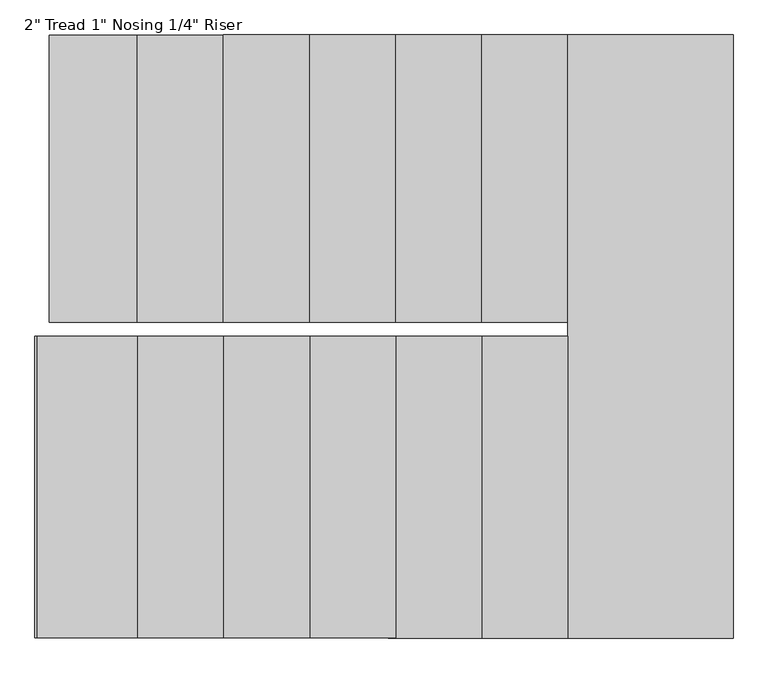
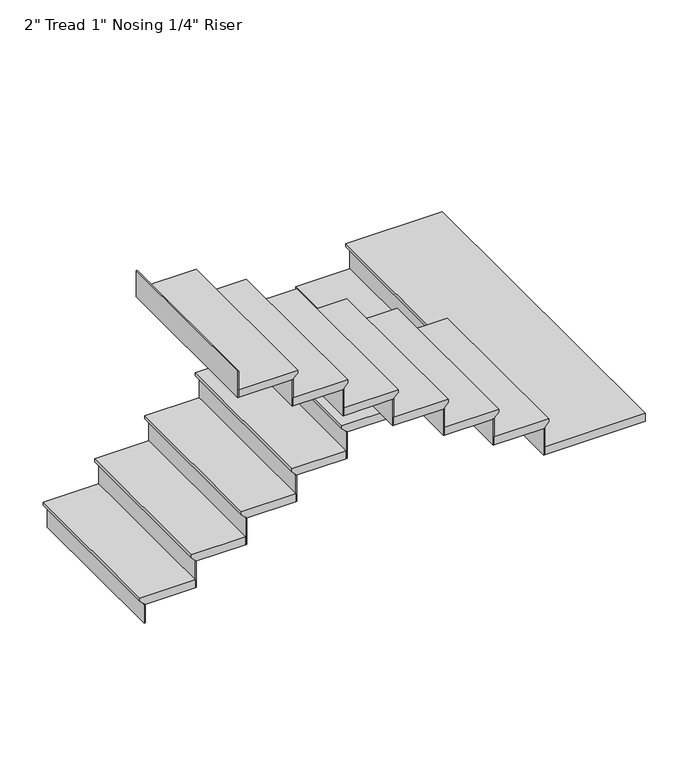
"""IFC4 building model written with IfcOpenShell, lengths in millimetres: stair flight geometry."""

from ifc_helpers import new_model, si_unit, origin, place, context, project, spatial, faceted_brep, source, transform, mapped, element, save


def stair_flight_cd9d6a89(model_context):
    return source(origin(), model_context, "Body", "Brep", [
        faceted_brep([(-1167.6638307, -167.7482799, 9751.4833333), (-1167.6638307, -167.7482799, 9770.5333333), (-1167.6638307, 848.2517201, 9770.5333333), (-1167.6638307, 848.2517201, 9751.4833333), (-1142.2638307, -167.7482799, 9726.0833333), (-1142.2638307, 848.2517201, 9726.0833333), (-831.1138307, -167.7482799, 9770.5333333), (-831.1138307, 848.2517201, 9770.5333333), (-1142.2638307, 848.2517201, 9719.7333333), (-831.1138307, 848.2517201, 9719.7333333), (-831.1138307, -167.7482799, 9719.7333333), (-1142.2638307, -167.7482799, 9719.7333333)], [[[0, 1, 2, 3]], [[4, 0, 3, 5]], [[2, 1, 6, 7]], [[8, 9, 10, 11]], [[2, 7, 9, 8, 5, 3]], [[8, 11, 4, 5]], [[6, 1, 0, 4, 11, 10]], [[7, 6, 10, 9]]]),
        faceted_brep([(-1142.2638307, -167.7482799, 9719.7333333), (-1142.2638307, -167.7482799, 9601.2), (-1135.9138307, -167.7482799, 9601.2), (-1135.9138307, -167.7482799, 9719.7333333), (-1142.2638307, 848.2517201, 9719.7333333), (-1135.9138307, 848.2517201, 9719.7333333), (-1135.9138307, 848.2517201, 9601.2), (-1142.2638307, 848.2517201, 9601.2)], [[[0, 1, 2, 3]], [[4, 5, 6, 7]], [[1, 0, 4, 7]], [[2, 1, 7, 6]], [[3, 2, 6, 5]], [[0, 3, 5, 4]]]),
        faceted_brep([(-831.1138307, -167.7482799, 9889.0666667), (-831.1138307, -167.7482799, 9719.7333333), (-824.7638307, -167.7482799, 9719.7333333), (-824.7638307, -167.7482799, 9889.0666667), (-831.1138307, 848.2517201, 9889.0666667), (-824.7638307, 848.2517201, 9889.0666667), (-824.7638307, 848.2517201, 9719.7333333), (-831.1138307, 848.2517201, 9719.7333333)], [[[0, 1, 2, 3]], [[4, 5, 6, 7]], [[1, 0, 4, 7]], [[2, 1, 7, 6]], [[3, 2, 6, 5]], [[0, 3, 5, 4]]]),
        faceted_brep([(-856.5138307, 848.2517201, 9939.8666667), (-856.5138307, -167.7482799, 9939.8666667), (-526.3138307, -167.7482799, 9939.8666667), (-526.3138307, 848.2517201, 9939.8666667), (-831.1138307, 848.2517201, 9889.0666667), (-526.3138307, 848.2517201, 9889.0666667), (-526.3138307, -167.7482799, 9889.0666667), (-831.1138307, -167.7482799, 9889.0666667), (-831.1138307, 848.2517201, 9895.4166667), (-856.5138307, 848.2517201, 9920.8166667), (-831.1138307, -167.7482799, 9895.4166667), (-856.5138307, -167.7482799, 9920.8166667)], [[[0, 1, 2, 3]], [[4, 5, 6, 7]], [[0, 3, 5, 4, 8, 9]], [[4, 7, 10, 8]], [[2, 1, 11, 10, 7, 6]], [[3, 2, 6, 5]], [[11, 1, 0, 9]], [[10, 11, 9, 8]]]),
        faceted_brep([(-526.3138307, -167.7482799, 10058.4), (-526.3138307, -167.7482799, 9889.0666667), (-519.9638307, -167.7482799, 9889.0666667), (-519.9638307, -167.7482799, 10058.4), (-526.3138307, 848.2517201, 10058.4), (-519.9638307, 848.2517201, 10058.4), (-519.9638307, 848.2517201, 9889.0666667), (-526.3138307, 848.2517201, 9889.0666667)], [[[0, 1, 2, 3]], [[4, 5, 6, 7]], [[1, 0, 4, 7]], [[2, 1, 7, 6]], [[3, 2, 6, 5]], [[0, 3, 5, 4]]]),
        faceted_brep([(-551.7138307, 848.2517201, 10109.2), (-551.7138307, -167.7482799, 10109.2), (-221.5138307, -167.7482799, 10109.2), (-221.5138307, 848.2517201, 10109.2), (-526.3138307, 848.2517201, 10058.4), (-221.5138307, 848.2517201, 10058.4), (-221.5138307, -167.7482799, 10058.4), (-526.3138307, -167.7482799, 10058.4), (-526.3138307, 848.2517201, 10064.75), (-551.7138307, 848.2517201, 10090.15), (-526.3138307, -167.7482799, 10064.75), (-551.7138307, -167.7482799, 10090.15)], [[[0, 1, 2, 3]], [[4, 5, 6, 7]], [[0, 3, 5, 4, 8, 9]], [[4, 7, 10, 8]], [[2, 1, 11, 10, 7, 6]], [[3, 2, 6, 5]], [[11, 1, 0, 9]], [[10, 11, 9, 8]]]),
        faceted_brep([(-221.5138307, -167.7482799, 10227.7333333), (-221.5138307, -167.7482799, 10058.4), (-215.1638307, -167.7482799, 10058.4), (-215.1638307, -167.7482799, 10227.7333333), (-221.5138307, 848.2517201, 10227.7333333), (-215.1638307, 848.2517201, 10227.7333333), (-215.1638307, 848.2517201, 10058.4), (-221.5138307, 848.2517201, 10058.4)], [[[0, 1, 2, 3]], [[4, 5, 6, 7]], [[1, 0, 4, 7]], [[2, 1, 7, 6]], [[3, 2, 6, 5]], [[0, 3, 5, 4]]]),
        faceted_brep([(-246.9138307, 848.2517201, 10278.5333333), (-246.9138307, -167.7482799, 10278.5333333), (83.2861693, -167.7482799, 10278.5333333), (83.2861693, 848.2517201, 10278.5333333), (-221.5138307, 848.2517201, 10227.7333333), (83.2861693, 848.2517201, 10227.7333333), (83.2861693, -167.7482799, 10227.7333333), (-221.5138307, -167.7482799, 10227.7333333), (-221.5138307, 848.2517201, 10234.0833333), (-246.9138307, 848.2517201, 10259.4833333), (-221.5138307, -167.7482799, 10234.0833333), (-246.9138307, -167.7482799, 10259.4833333)], [[[0, 1, 2, 3]], [[4, 5, 6, 7]], [[0, 3, 5, 4, 8, 9]], [[4, 7, 10, 8]], [[2, 1, 11, 10, 7, 6]], [[3, 2, 6, 5]], [[11, 1, 0, 9]], [[10, 11, 9, 8]]]),
        faceted_brep([(83.2861693, -167.7482799, 10397.0666667), (83.2861693, -167.7482799, 10227.7333333), (89.6361693, -167.7482799, 10227.7333333), (89.6361693, -167.7482799, 10397.0666667), (83.2861693, 848.2517201, 10397.0666667), (89.6361693, 848.2517201, 10397.0666667), (89.6361693, 848.2517201, 10227.7333333), (83.2861693, 848.2517201, 10227.7333333)], [[[0, 1, 2, 3]], [[4, 5, 6, 7]], [[1, 0, 4, 7]], [[2, 1, 7, 6]], [[3, 2, 6, 5]], [[0, 3, 5, 4]]]),
        faceted_brep([(57.8861693, 848.2517201, 10447.8666667), (57.8861693, -167.7482799, 10447.8666667), (388.0861693, -167.7482799, 10447.8666667), (388.0861693, 848.2517201, 10447.8666667), (83.2861693, 848.2517201, 10397.0666667), (388.0861693, 848.2517201, 10397.0666667), (388.0861693, -167.7482799, 10397.0666667), (83.2861693, -167.7482799, 10397.0666667), (83.2861693, 848.2517201, 10403.4166667), (57.8861693, 848.2517201, 10428.8166667), (83.2861693, -167.7482799, 10403.4166667), (57.8861693, -167.7482799, 10428.8166667)], [[[0, 1, 2, 3]], [[4, 5, 6, 7]], [[0, 3, 5, 4, 8, 9]], [[4, 7, 10, 8]], [[2, 1, 11, 10, 7, 6]], [[3, 2, 6, 5]], [[11, 1, 0, 9]], [[10, 11, 9, 8]]]),
        faceted_brep([(388.0861693, -167.7482799, 10566.4), (388.0861693, -167.7482799, 10397.0666667), (394.4361693, -167.7482799, 10397.0666667), (394.4361693, -167.7482799, 10566.4), (388.0861693, 848.2517201, 10566.4), (394.4361693, 848.2517201, 10566.4), (394.4361693, 848.2517201, 10397.0666667), (388.0861693, 848.2517201, 10397.0666667)], [[[0, 1, 2, 3]], [[4, 5, 6, 7]], [[1, 0, 4, 7]], [[2, 1, 7, 6]], [[3, 2, 6, 5]], [[0, 3, 5, 4]]]),
        faceted_brep([(362.6861693, 848.2517201, 10617.2), (362.6861693, -167.7482799, 10617.2), (692.8861693, -167.7482799, 10617.2), (692.8861693, 848.2517201, 10617.2), (388.0861693, 848.2517201, 10566.4), (692.8861693, 848.2517201, 10566.4), (692.8861693, -167.7482799, 10566.4), (388.0861693, -167.7482799, 10566.4), (388.0861693, 848.2517201, 10572.75), (362.6861693, 848.2517201, 10598.15), (388.0861693, -167.7482799, 10572.75), (362.6861693, -167.7482799, 10598.15)], [[[0, 1, 2, 3]], [[4, 5, 6, 7]], [[0, 3, 5, 4, 8, 9]], [[4, 7, 10, 8]], [[2, 1, 11, 10, 7, 6]], [[3, 2, 6, 5]], [[11, 1, 0, 9]], [[10, 11, 9, 8]]]),
        faceted_brep([(692.8861693, -167.7482799, 10735.7333333), (692.8861693, -167.7482799, 10566.4), (699.2361693, -167.7482799, 10566.4), (699.2361693, -167.7482799, 10735.7333333), (692.8861693, 848.2517201, 10735.7333333), (699.2361693, 848.2517201, 10735.7333333), (699.2361693, 848.2517201, 10566.4), (692.8861693, 848.2517201, 10566.4)], [[[0, 1, 2, 3]], [[4, 5, 6, 7]], [[1, 0, 4, 7]], [[2, 1, 7, 6]], [[3, 2, 6, 5]], [[0, 3, 5, 4]]]),
        faceted_brep([(642.0861693, -1285.3482799, 10786.5333333), (1251.6861693, -1285.3482799, 10786.5333333), (1251.6861693, 848.2517201, 10786.5333333), (667.4861693, 848.2517201, 10786.5333333), (667.4861693, -218.5482799, 10786.5333333), (642.0861693, -218.5482799, 10786.5333333), (1251.6861693, -1285.3482799, 10735.7333333), (642.0861693, -1285.3482799, 10735.7333333), (642.0861693, -218.5482799, 10735.7333333), (667.4861693, -218.5482799, 10735.7333333), (667.4861693, -167.7482799, 10735.7333333), (692.8861693, -167.7482799, 10735.7333333), (692.8861693, 848.2517201, 10735.7333333), (1251.6861693, 848.2517201, 10735.7333333), (692.8861693, 848.2517201, 10742.0833333), (667.4861693, 848.2517201, 10767.4833333), (692.8861693, -167.7482799, 10742.0833333), (667.4861693, -167.7482799, 10767.4833333)], [[[0, 1, 2, 3, 4, 5]], [[6, 7, 8, 9, 10, 11, 12, 13]], [[1, 0, 7, 6]], [[2, 1, 6, 13]], [[3, 2, 13, 12, 14, 15]], [[12, 11, 16, 14]], [[11, 10, 17, 16]], [[4, 3, 15, 17, 10, 9]], [[5, 4, 9, 8]], [[0, 5, 8, 7]], [[15, 14, 16, 17]]]),
        faceted_brep([(642.0861693, -218.5482799, 10905.0666667), (642.0861693, -218.5482799, 10735.7333333), (635.7361693, -218.5482799, 10735.7333333), (635.7361693, -218.5482799, 10905.0666667), (642.0861693, -1285.3482799, 10905.0666667), (635.7361693, -1285.3482799, 10905.0666667), (635.7361693, -1285.3482799, 10735.7333333), (642.0861693, -1285.3482799, 10735.7333333)], [[[0, 1, 2, 3]], [[4, 5, 6, 7]], [[1, 0, 4, 7]], [[2, 1, 7, 6]], [[3, 2, 6, 5]], [[0, 3, 5, 4]]]),
        faceted_brep([(667.4861693, -1285.3482799, 10955.8666667), (667.4861693, -218.5482799, 10955.8666667), (337.2861693, -218.5482799, 10955.8666667), (337.2861693, -1285.3482799, 10955.8666667), (642.0861693, -1285.3482799, 10905.0666667), (337.2861693, -1285.3482799, 10905.0666667), (337.2861693, -218.5482799, 10905.0666667), (642.0861693, -218.5482799, 10905.0666667), (642.0861693, -1285.3482799, 10911.4166667), (667.4861693, -1285.3482799, 10936.8166667), (642.0861693, -218.5482799, 10911.4166667), (667.4861693, -218.5482799, 10936.8166667)], [[[0, 1, 2, 3]], [[4, 5, 6, 7]], [[0, 3, 5, 4, 8, 9]], [[4, 7, 10, 8]], [[2, 1, 11, 10, 7, 6]], [[3, 2, 6, 5]], [[11, 1, 0, 9]], [[10, 11, 9, 8]]]),
        faceted_brep([(337.2861693, -218.5482799, 11074.4), (337.2861693, -218.5482799, 10905.0666667), (330.9361693, -218.5482799, 10905.0666667), (330.9361693, -218.5482799, 11074.4), (337.2861693, -1285.3482799, 11074.4), (330.9361693, -1285.3482799, 11074.4), (330.9361693, -1285.3482799, 10905.0666667), (337.2861693, -1285.3482799, 10905.0666667)], [[[0, 1, 2, 3]], [[4, 5, 6, 7]], [[1, 0, 4, 7]], [[2, 1, 7, 6]], [[3, 2, 6, 5]], [[0, 3, 5, 4]]]),
        faceted_brep([(362.6861693, -1285.3482799, 11125.2), (362.6861693, -218.5482799, 11125.2), (32.4861693, -218.5482799, 11125.2), (32.4861693, -1285.3482799, 11125.2), (337.2861693, -1285.3482799, 11074.4), (32.4861693, -1285.3482799, 11074.4), (32.4861693, -218.5482799, 11074.4), (337.2861693, -218.5482799, 11074.4), (337.2861693, -1285.3482799, 11080.75), (362.6861693, -1285.3482799, 11106.15), (337.2861693, -218.5482799, 11080.75), (362.6861693, -218.5482799, 11106.15)], [[[0, 1, 2, 3]], [[4, 5, 6, 7]], [[0, 3, 5, 4, 8, 9]], [[4, 7, 10, 8]], [[2, 1, 11, 10, 7, 6]], [[3, 2, 6, 5]], [[11, 1, 0, 9]], [[10, 11, 9, 8]]]),
        faceted_brep([(32.4861693, -218.5482799, 11243.7333333), (32.4861693, -218.5482799, 11074.4), (26.1361693, -218.5482799, 11074.4), (26.1361693, -218.5482799, 11243.7333333), (32.4861693, -1285.3482799, 11243.7333333), (26.1361693, -1285.3482799, 11243.7333333), (26.1361693, -1285.3482799, 11074.4), (32.4861693, -1285.3482799, 11074.4)], [[[0, 1, 2, 3]], [[4, 5, 6, 7]], [[1, 0, 4, 7]], [[2, 1, 7, 6]], [[3, 2, 6, 5]], [[0, 3, 5, 4]]]),
        faceted_brep([(57.8861693, -1285.3482799, 11294.5333333), (57.8861693, -218.5482799, 11294.5333333), (-272.3138307, -218.5482799, 11294.5333333), (-272.3138307, -1285.3482799, 11294.5333333), (32.4861693, -1285.3482799, 11243.7333333), (-272.3138307, -1285.3482799, 11243.7333333), (-272.3138307, -218.5482799, 11243.7333333), (32.4861693, -218.5482799, 11243.7333333), (32.4861693, -1285.3482799, 11250.0833333), (57.8861693, -1285.3482799, 11275.4833333), (32.4861693, -218.5482799, 11250.0833333), (57.8861693, -218.5482799, 11275.4833333)], [[[0, 1, 2, 3]], [[4, 5, 6, 7]], [[0, 3, 5, 4, 8, 9]], [[4, 7, 10, 8]], [[2, 1, 11, 10, 7, 6]], [[3, 2, 6, 5]], [[11, 1, 0, 9]], [[10, 11, 9, 8]]]),
        faceted_brep([(-272.3138307, -218.5482799, 11413.0666667), (-272.3138307, -218.5482799, 11243.7333333), (-278.6638307, -218.5482799, 11243.7333333), (-278.6638307, -218.5482799, 11413.0666667), (-272.3138307, -1285.3482799, 11413.0666667), (-278.6638307, -1285.3482799, 11413.0666667), (-278.6638307, -1285.3482799, 11243.7333333), (-272.3138307, -1285.3482799, 11243.7333333)], [[[0, 1, 2, 3]], [[4, 5, 6, 7]], [[1, 0, 4, 7]], [[2, 1, 7, 6]], [[3, 2, 6, 5]], [[0, 3, 5, 4]]]),
        faceted_brep([(-246.9138307, -1285.3482799, 11463.8666667), (-246.9138307, -218.5482799, 11463.8666667), (-577.1138307, -218.5482799, 11463.8666667), (-577.1138307, -1285.3482799, 11463.8666667), (-272.3138307, -1285.3482799, 11413.0666667), (-577.1138307, -1285.3482799, 11413.0666667), (-577.1138307, -218.5482799, 11413.0666667), (-272.3138307, -218.5482799, 11413.0666667), (-272.3138307, -1285.3482799, 11419.4166667), (-246.9138307, -1285.3482799, 11444.8166667), (-272.3138307, -218.5482799, 11419.4166667), (-246.9138307, -218.5482799, 11444.8166667)], [[[0, 1, 2, 3]], [[4, 5, 6, 7]], [[0, 3, 5, 4, 8, 9]], [[4, 7, 10, 8]], [[2, 1, 11, 10, 7, 6]], [[3, 2, 6, 5]], [[11, 1, 0, 9]], [[10, 11, 9, 8]]]),
        faceted_brep([(-577.1138307, -218.5482799, 11582.4), (-577.1138307, -218.5482799, 11413.0666667), (-583.4638307, -218.5482799, 11413.0666667), (-583.4638307, -218.5482799, 11582.4), (-577.1138307, -1285.3482799, 11582.4), (-583.4638307, -1285.3482799, 11582.4), (-583.4638307, -1285.3482799, 11413.0666667), (-577.1138307, -1285.3482799, 11413.0666667)], [[[0, 1, 2, 3]], [[4, 5, 6, 7]], [[1, 0, 4, 7]], [[2, 1, 7, 6]], [[3, 2, 6, 5]], [[0, 3, 5, 4]]]),
        faceted_brep([(-551.7138307, -1285.3482799, 11633.2), (-551.7138307, -218.5482799, 11633.2), (-881.9138307, -218.5482799, 11633.2), (-881.9138307, -1285.3482799, 11633.2), (-577.1138307, -1285.3482799, 11582.4), (-881.9138307, -1285.3482799, 11582.4), (-881.9138307, -218.5482799, 11582.4), (-577.1138307, -218.5482799, 11582.4), (-577.1138307, -1285.3482799, 11588.75), (-551.7138307, -1285.3482799, 11614.15), (-577.1138307, -218.5482799, 11588.75), (-551.7138307, -218.5482799, 11614.15)], [[[0, 1, 2, 3]], [[4, 5, 6, 7]], [[0, 3, 5, 4, 8, 9]], [[4, 7, 10, 8]], [[2, 1, 11, 10, 7, 6]], [[3, 2, 6, 5]], [[11, 1, 0, 9]], [[10, 11, 9, 8]]]),
        faceted_brep([(-881.9138307, -218.5482799, 11751.7333333), (-881.9138307, -218.5482799, 11582.4), (-888.2638307, -218.5482799, 11582.4), (-888.2638307, -218.5482799, 11751.7333333), (-881.9138307, -1285.3482799, 11751.7333333), (-888.2638307, -1285.3482799, 11751.7333333), (-888.2638307, -1285.3482799, 11582.4), (-881.9138307, -1285.3482799, 11582.4)], [[[0, 1, 2, 3]], [[4, 5, 6, 7]], [[1, 0, 4, 7]], [[2, 1, 7, 6]], [[3, 2, 6, 5]], [[0, 3, 5, 4]]]),
        faceted_brep([(-1212.1138307, -218.5482799, 11921.0666667), (-1212.1138307, -218.5482799, 11751.7333333), (-1218.4638307, -218.5482799, 11751.7333333), (-1218.4638307, -218.5482799, 11921.0666667), (-1212.1138307, -1285.3482799, 11921.0666667), (-1218.4638307, -1285.3482799, 11921.0666667), (-1218.4638307, -1285.3482799, 11751.7333333), (-1212.1138307, -1285.3482799, 11751.7333333)], [[[0, 1, 2, 3]], [[4, 5, 6, 7]], [[1, 0, 4, 7]], [[2, 1, 7, 6]], [[3, 2, 6, 5]], [[0, 3, 5, 4]]]),
        faceted_brep([(-856.5138307, -1285.3482799, 11802.5333333), (-856.5138307, -218.5482799, 11802.5333333), (-1212.1138307, -218.5482799, 11802.5333333), (-1212.1138307, -1285.3482799, 11802.5333333), (-881.9138307, -1285.3482799, 11751.7333333), (-1212.1138307, -1285.3482799, 11751.7333333), (-1212.1138307, -218.5482799, 11751.7333333), (-881.9138307, -218.5482799, 11751.7333333), (-881.9138307, -1285.3482799, 11758.0833333), (-856.5138307, -1285.3482799, 11783.4833333), (-881.9138307, -218.5482799, 11758.0833333), (-856.5138307, -218.5482799, 11783.4833333)], [[[0, 1, 2, 3]], [[4, 5, 6, 7]], [[0, 3, 5, 4, 8, 9]], [[4, 7, 10, 8]], [[2, 1, 11, 10, 7, 6]], [[3, 2, 6, 5]], [[11, 1, 0, 9]], [[10, 11, 9, 8]]]),
    ])


if __name__ == "__main__":
    model = new_model("IFC4")
    model_context = context("Model", 3, world=origin())
    ifc_project = project(units=[si_unit("LENGTHUNIT", "METRE", prefix="MILLI")], contexts=[model_context])
    site = spatial("IfcSite", under=ifc_project)
    building = spatial("IfcBuilding", under=site)
    placement = place(None, origin())
    stair_flight_shape = stair_flight_cd9d6a89(model_context)
    element("IfcStairFlight", 1, ObjectType="2\" Tread 1\" Nosing 1/4\" Riser", at=placement, inside=building, context=model_context, shape_type="MappedRepresentation", body=[
        mapped(stair_flight_shape, transform((0.0, 0.0, 0.0), x_axis=(1.0, 0.0, 0.0), y_axis=(0.0, 1.0, 0.0), z_axis=(0.0, 0.0, 1.0))),
    ])
    save(model, "model.ifc")
